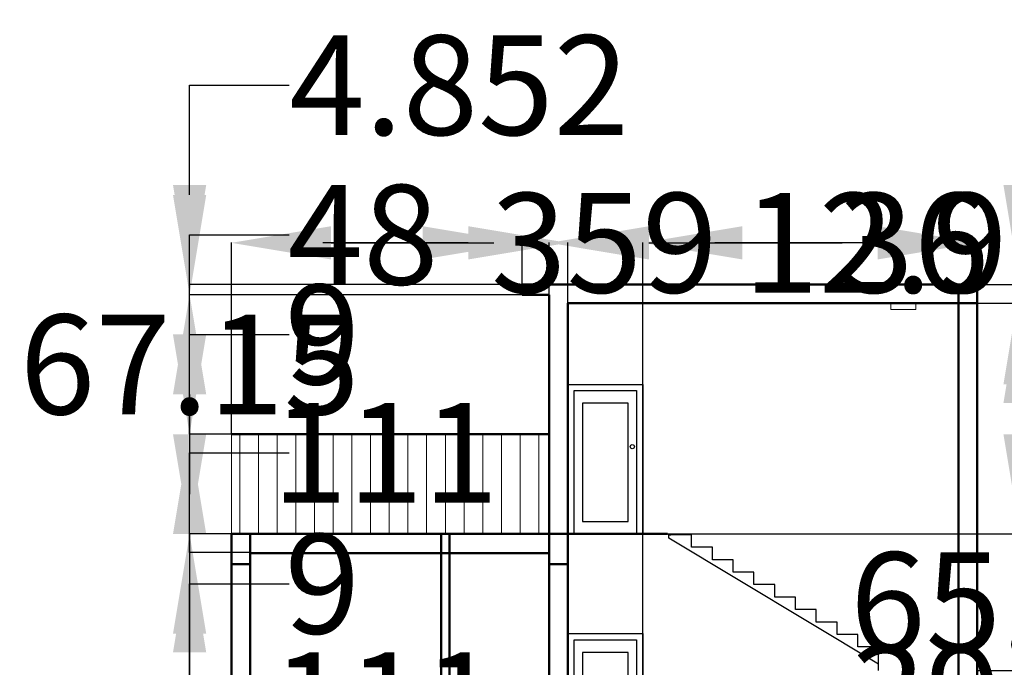
# Model space of a CAD drawing. Units: inches. Extents: x 131 to 858, y -65 to 554.
# Tile 3 of 4: x 131 to 605, y 242 to 554. Entities that reach past the tile are written whole.
import ezdxf

# ---------------------------------------------------------------- set-up
doc = ezdxf.new("R2010")
doc.units = ezdxf.units.IN
doc.header["$MEASUREMENT"] = 0
for name, color, linetype, lineweight in [('A-ANNO-DIMS', 2, 'Continuous', 18), ('A-DOOR', 4, 'Continuous', 25), ('A-EQPM', 8, 'Continuous', 18), ('A-FLOR-HRAL', 4, 'Continuous', 18), ('A-FLOR-STRS', 3, 'Continuous', 25), ('A-SECT', 7, 'Continuous', 50)]:
    doc.layers.add(name, color=color, linetype=linetype, lineweight=lineweight)
doc.styles.get("Standard").update_dxf_attribs({"font": 'arial.ttf'})
doc.dimstyles.get("Standard").update_dxf_attribs({"dimtxt": 48, "dimasz": 48, "dimexe": 0.18, "dimexo": 0.0625, "dimgap": 0.09, "dimtad": 0, "dimtih": 1, "dimtoh": 1, "dimdec": 0, "dimrnd": 72, "dimzin": 0, "dimdsep": 46, "dimlunit": 3, "dimtxsty": 'Standard', "dimcen": 0.09, "dimadec": 0, "dimazin": 0, "dimtfac": 1, "dimtdec": 0, "dimtofl": 0, "dimtmove": 0, "dimatfit": 3, "dimfxl": 1, "dimtolj": 1, "dimtzin": 0, "dimarcsym": 0})

# ---------------------------------------------------------------- blocks, each defined once
blk = doc.blocks.new('*U3')
blk.add_lwpolyline([(3.12, 0.01), (0.12, 0.01), (0.12, 72.01), (36.12, 72.01), (36.12, 0.01), (33.12, 0.01)])
for points in [[(33.12, 68.99), (33.12, 0.01), (3.12, 0.01), (3.12, 68.99)], [(29.12, 6.01), (29.12, 62.99), (7.12, 62.99), (7.12, 6.01)]]:
    blk.add_lwpolyline(points, close=True)
blk.add_circle((31.12, 42.01), 1)
blk = doc.blocks.new('*D4')
at = {"layer": 'A-ANNO-DIMS', "color": 0, "lineweight": -2, "transparency": 16777216}
for p, q in [((233.01, 354.61), (233.01, 446.83)), ((281.01, 446.65), (359.38, 446.65)), ((544.04, 446.65), (465.68, 446.65)), ((592.04, 426.61), (592.04, 446.83))]:
    blk.add_line(p, q, dxfattribs=at)
at = {"layer": 'A-ANNO-DIMS', "color": 0, "transparency": 16777216}
for points in [[(281.01, 454.65), (281.01, 438.65), (233.01, 446.65)], [(544.04, 454.65), (544.04, 438.65), (592.04, 446.65)]]:
    blk.add_solid(points, dxfattribs=at)
at = {"layer": 'Defpoints', "color": 0, "transparency": 16777216}
for p in [(592.04, 446.65), (592.04, 426.55), (233.01, 354.55)]:
    blk.add_point(p, dxfattribs=at)
at = {"layer": 'A-ANNO-DIMS', "color": 0, "transparency": 16777216, "insert": (412.53, 446.65), "char_height": 48, "attachment_point": 5}
blk.add_mtext('\\A1;359', dxfattribs=at)
blk = doc.blocks.new('*D5')
at = {"layer": 'A-ANNO-DIMS', "color": 0, "lineweight": -2, "transparency": 16777216}
for p, q in [((325.03, 446.65), (277.03, 446.65)), ((373.03, 426.61), (373.03, 446.83)), ((386.01, 421.76), (386.01, 446.83)), ((434.01, 446.65), (482.01, 446.65))]:
    blk.add_line(p, q, dxfattribs=at)
at = {"layer": 'A-ANNO-DIMS', "color": 0, "transparency": 16777216}
for points in [[(325.03, 454.65), (325.03, 438.65), (373.03, 446.65)], [(434.01, 454.65), (434.01, 438.65), (386.01, 446.65)]]:
    blk.add_solid(points, dxfattribs=at)
at = {"layer": 'Defpoints', "color": 0, "transparency": 16777216}
for p in [(386.01, 446.65), (373.03, 426.55), (386.01, 421.7)]:
    blk.add_point(p, dxfattribs=at)
at = {"layer": 'A-ANNO-DIMS', "color": 0, "transparency": 16777216, "insert": (579.38, 446.65), "char_height": 48, "attachment_point": 5}
blk.add_mtext('\\A1;12.984', dxfattribs=at)
blk = doc.blocks.new('*D14')
at = {"layer": 'A-ANNO-DIMS', "color": 0, "lineweight": -2, "transparency": 16777216}
for p, q in [((592.11, 426.55), (612.82, 426.55)), ((612.64, 378.55), (612.64, 253.56)), ((612.64, 79.34), (612.64, 204.33)), ((233.08, 31.34), (612.82, 31.34))]:
    blk.add_line(p, q, dxfattribs=at)
at = {"layer": 'A-ANNO-DIMS', "color": 0, "transparency": 16777216}
for points in [[(604.64, 378.55), (620.64, 378.55), (612.64, 426.55)], [(604.64, 79.34), (620.64, 79.34), (612.64, 31.34)]]:
    blk.add_solid(points, dxfattribs=at)
at = {"layer": 'Defpoints', "color": 0, "transparency": 16777216}
for p in [(592.04, 426.55), (612.64, 426.55), (233.01, 31.34)]:
    blk.add_point(p, dxfattribs=at)
at = {"layer": 'A-ANNO-DIMS', "color": 0, "transparency": 16777216, "insert": (612.64, 228.94), "char_height": 48, "attachment_point": 5}
blk.add_mtext('\\A1;395.2', dxfattribs=at)
blk = doc.blocks.new('*D23')
at = {"layer": 'A-ANNO-DIMS', "color": 0, "lineweight": -2, "transparency": 16777216}
for p, q in [((212.91, 177.55), (212.91, 225.55)), ((212.91, 225.55), (260.91, 225.55)), ((241.95, 177.55), (212.73, 177.55)), ((212.91, 114.55), (212.91, 129.55)), ((232.95, 66.55), (212.73, 66.55))]:
    blk.add_line(p, q, dxfattribs=at)
at = {"layer": 'A-ANNO-DIMS', "color": 0, "transparency": 16777216}
for points in [[(204.91, 129.55), (220.91, 129.55), (212.91, 177.55)], [(204.91, 114.55), (220.91, 114.55), (212.91, 66.55)]]:
    blk.add_solid(points, dxfattribs=at)
at = {"layer": 'Defpoints', "color": 0, "transparency": 16777216}
for p in [(212.91, 177.55), (242.01, 177.55), (233.01, 66.55)]:
    blk.add_point(p, dxfattribs=at)
at = {"layer": 'A-ANNO-DIMS', "color": 0, "transparency": 16777216, "insert": (307.14, 225.55), "char_height": 48, "attachment_point": 5}
blk.add_mtext('\\A1;111', dxfattribs=at)
blk = doc.blocks.new('*D24')
at = {"layer": 'A-ANNO-DIMS', "color": 0, "lineweight": -2, "transparency": 16777216}
for p, q in [((212.91, 234.55), (212.91, 282.55)), ((212.91, 282.55), (260.91, 282.55)), ((232.95, 186.55), (212.73, 186.55)), ((241.95, 177.55), (212.73, 177.55)), ((212.91, 129.55), (212.91, 81.55))]:
    blk.add_line(p, q, dxfattribs=at)
at = {"layer": 'A-ANNO-DIMS', "color": 0, "transparency": 16777216}
for points in [[(204.91, 234.55), (220.91, 234.55), (212.91, 186.55)], [(204.91, 129.55), (220.91, 129.55), (212.91, 177.55)]]:
    blk.add_solid(points, dxfattribs=at)
at = {"layer": 'Defpoints', "color": 0, "transparency": 16777216}
for p in [(212.91, 186.55), (233.01, 186.55), (242.01, 177.55)]:
    blk.add_point(p, dxfattribs=at)
at = {"layer": 'A-ANNO-DIMS', "color": 0, "transparency": 16777216, "insert": (276.79, 282.55), "char_height": 48, "attachment_point": 5}
blk.add_mtext('\\A1;9', dxfattribs=at)
blk = doc.blocks.new('*D25')
at = {"layer": 'A-ANNO-DIMS', "color": 0, "lineweight": -2, "transparency": 16777216}
for p, q in [((212.91, 297.55), (212.91, 345.55)), ((212.91, 345.55), (260.91, 345.55)), ((241.95, 297.55), (212.73, 297.55)), ((212.91, 234.55), (212.91, 249.55)), ((232.95, 186.55), (212.73, 186.55))]:
    blk.add_line(p, q, dxfattribs=at)
at = {"layer": 'A-ANNO-DIMS', "color": 0, "transparency": 16777216}
for points in [[(204.91, 249.55), (220.91, 249.55), (212.91, 297.55)], [(204.91, 234.55), (220.91, 234.55), (212.91, 186.55)]]:
    blk.add_solid(points, dxfattribs=at)
at = {"layer": 'Defpoints', "color": 0, "transparency": 16777216}
for p in [(212.91, 297.55), (242.01, 297.55), (233.01, 186.55)]:
    blk.add_point(p, dxfattribs=at)
at = {"layer": 'A-ANNO-DIMS', "color": 0, "transparency": 16777216, "insert": (307.14, 345.55), "char_height": 48, "attachment_point": 5}
blk.add_mtext('\\A1;111', dxfattribs=at)
blk = doc.blocks.new('*D26')
at = {"layer": 'A-ANNO-DIMS', "color": 0, "lineweight": -2, "transparency": 16777216}
for p, q in [((212.91, 354.55), (212.91, 402.55)), ((212.91, 402.55), (260.91, 402.55)), ((232.95, 306.55), (212.73, 306.55)), ((241.95, 297.55), (212.73, 297.55)), ((212.91, 249.55), (212.91, 201.55))]:
    blk.add_line(p, q, dxfattribs=at)
at = {"layer": 'A-ANNO-DIMS', "color": 0, "transparency": 16777216}
for points in [[(204.91, 354.55), (220.91, 354.55), (212.91, 306.55)], [(204.91, 249.55), (220.91, 249.55), (212.91, 297.55)]]:
    blk.add_solid(points, dxfattribs=at)
at = {"layer": 'Defpoints', "color": 0, "transparency": 16777216}
for p in [(212.91, 306.55), (233.01, 306.55), (242.01, 297.55)]:
    blk.add_point(p, dxfattribs=at)
at = {"layer": 'A-ANNO-DIMS', "color": 0, "transparency": 16777216, "insert": (276.79, 402.55), "char_height": 48, "attachment_point": 5}
blk.add_mtext('\\A1;9', dxfattribs=at)
blk = doc.blocks.new('*D27')
at = {"layer": 'A-ANNO-DIMS', "color": 0, "lineweight": -2, "transparency": 16777216}
for p, q in [((212.91, 402.55), (212.91, 450.55)), ((212.91, 450.55), (260.91, 450.55)), ((232.95, 354.55), (212.73, 354.55)), ((232.95, 306.55), (212.73, 306.55)), ((212.91, 258.55), (212.91, 210.55))]:
    blk.add_line(p, q, dxfattribs=at)
at = {"layer": 'A-ANNO-DIMS', "color": 0, "transparency": 16777216}
for points in [[(204.91, 402.55), (220.91, 402.55), (212.91, 354.55)], [(204.91, 258.55), (220.91, 258.55), (212.91, 306.55)]]:
    blk.add_solid(points, dxfattribs=at)
at = {"layer": 'Defpoints', "color": 0, "transparency": 16777216}
for p in [(212.91, 354.55), (233.01, 354.55), (233.01, 306.55)]:
    blk.add_point(p, dxfattribs=at)
at = {"layer": 'A-ANNO-DIMS', "color": 0, "transparency": 16777216, "insert": (296.4, 450.55), "char_height": 48, "attachment_point": 5}
blk.add_mtext('\\A1;48', dxfattribs=at)
blk = doc.blocks.new('*D28')
at = {"layer": 'A-ANNO-DIMS', "color": 0, "lineweight": -2, "transparency": 16777216}
for p, q in [((212.914446, 469.69966), (212.914446, 517.69966)), ((372.967658, 421.69966), (212.734446, 421.69966)), ((232.951946, 354.551418), (212.734446, 354.551418)), ((212.914446, 306.551418), (212.914446, 258.551418))]:
    blk.add_line(p, q, dxfattribs=at)
at = {"layer": 'A-ANNO-DIMS', "color": 0, "transparency": 16777216}
for points in [[(204.914446, 469.69966), (220.914446, 469.69966), (212.914446, 421.69966)], [(204.914446, 306.551418), (220.914446, 306.551418), (212.914446, 354.551418)]]:
    blk.add_solid(points, dxfattribs=at)
at = {"layer": 'Defpoints', "color": 0, "transparency": 16777216}
for p in [(212.914446, 421.69966), (373.030158, 421.69966), (233.014446, 354.551418)]:
    blk.add_point(p, dxfattribs=at)
at = {"layer": 'A-ANNO-DIMS', "color": 0, "transparency": 16777216, "insert": (212.914446, 388.125539), "char_height": 48, "attachment_point": 5}
blk.add_mtext('\\A1;67.15', dxfattribs=at)
blk = doc.blocks.new('*D29')
at = {"layer": 'A-ANNO-DIMS', "color": 0, "lineweight": -2, "transparency": 16777216}
for p, q in [((212.91, 474.55), (212.91, 522.55)), ((212.91, 522.55), (260.91, 522.55)), ((372.97, 426.55), (212.73, 426.55)), ((372.97, 421.7), (212.73, 421.7)), ((212.91, 373.7), (212.91, 325.7))]:
    blk.add_line(p, q, dxfattribs=at)
at = {"layer": 'A-ANNO-DIMS', "color": 0, "transparency": 16777216}
for points in [[(204.91, 474.55), (220.91, 474.55), (212.91, 426.55)], [(204.91, 373.7), (220.91, 373.7), (212.91, 421.7)]]:
    blk.add_solid(points, dxfattribs=at)
at = {"layer": 'Defpoints', "color": 0, "transparency": 16777216}
for p in [(212.91, 426.55), (373.03, 426.55), (373.03, 421.7)]:
    blk.add_point(p, dxfattribs=at)
at = {"layer": 'A-ANNO-DIMS', "color": 0, "transparency": 16777216, "insert": (342.71, 522.55), "char_height": 48, "attachment_point": 5}
blk.add_mtext('\\A1;4.852', dxfattribs=at)
blk = doc.blocks.new('*D30')
at = {"layer": 'A-ANNO-DIMS', "color": 0, "lineweight": -2, "transparency": 16777216}
for p, q in [((612.64, 417.55), (612.64, 465.55)), ((612.64, 465.55), (660.64, 465.55)), ((592.11, 417.55), (612.82, 417.55)), ((612.64, 354.55), (612.64, 369.55)), ((443.08, 306.55), (612.82, 306.55))]:
    blk.add_line(p, q, dxfattribs=at)
at = {"layer": 'A-ANNO-DIMS', "color": 0, "transparency": 16777216}
for points in [[(604.64, 369.55), (620.64, 369.55), (612.64, 417.55)], [(604.64, 354.55), (620.64, 354.55), (612.64, 306.55)]]:
    blk.add_solid(points, dxfattribs=at)
at = {"layer": 'Defpoints', "color": 0, "transparency": 16777216}
for p in [(592.04, 417.55), (612.64, 417.55), (443.01, 306.55)]:
    blk.add_point(p, dxfattribs=at)
at = {"layer": 'A-ANNO-DIMS', "color": 0, "transparency": 16777216, "insert": (706.86, 465.55), "char_height": 48, "attachment_point": 5}
blk.add_mtext('\\A1;111', dxfattribs=at)
blk = doc.blocks.new('*D31')
at = {"layer": 'A-ANNO-DIMS', "color": 0, "lineweight": -2, "transparency": 16777216}
for p, q in [((612.64, 474.55), (612.64, 522.55)), ((612.64, 522.55), (660.64, 522.55)), ((592.11, 426.55), (612.82, 426.55)), ((592.11, 417.55), (612.82, 417.55)), ((612.64, 369.55), (612.64, 321.55))]:
    blk.add_line(p, q, dxfattribs=at)
at = {"layer": 'A-ANNO-DIMS', "color": 0, "transparency": 16777216}
for points in [[(604.64, 474.55), (620.64, 474.55), (612.64, 426.55)], [(604.64, 369.55), (620.64, 369.55), (612.64, 417.55)]]:
    blk.add_solid(points, dxfattribs=at)
at = {"layer": 'Defpoints', "color": 0, "transparency": 16777216}
for p in [(592.04, 426.55), (612.64, 426.55), (592.04, 417.55)]:
    blk.add_point(p, dxfattribs=at)
at = {"layer": 'A-ANNO-DIMS', "color": 0, "transparency": 16777216, "insert": (676.51, 522.55), "char_height": 48, "attachment_point": 5}
blk.add_mtext('\\A1;9', dxfattribs=at)
blk = doc.blocks.new('*D32')
at = {"layer": 'A-ANNO-DIMS', "color": 0, "lineweight": -2, "transparency": 16777216}
for p, q in [((347.01, 446.65), (299.01, 446.65)), ((395.01, 138.61), (395.01, 446.83)), ((431.01, 138.61), (431.01, 446.83)), ((479.01, 446.65), (527.01, 446.65))]:
    blk.add_line(p, q, dxfattribs=at)
at = {"layer": 'A-ANNO-DIMS', "color": 0, "transparency": 16777216}
for points in [[(347.01, 454.65), (347.01, 438.65), (395.01, 446.65)], [(479.01, 454.65), (479.01, 438.65), (431.01, 446.65)]]:
    blk.add_solid(points, dxfattribs=at)
at = {"layer": 'Defpoints', "color": 0, "transparency": 16777216}
for p in [(431.01, 446.65), (395.01, 138.55), (431.01, 138.55)]:
    blk.add_point(p, dxfattribs=at)
at = {"layer": 'A-ANNO-DIMS', "color": 0, "transparency": 16777216, "insert": (561.45, 446.65), "char_height": 48, "attachment_point": 5}
blk.add_mtext('\\A1;36', dxfattribs=at)
blk = doc.blocks.new('*D42')
at = {"layer": 'A-ANNO-DIMS', "color": 0, "lineweight": -2, "transparency": 16777216}
for p, q in [((612.64, 240.89), (612.64, 288.89)), ((612.64, 288.89), (660.64, 288.89)), ((592.6, 240.89), (612.82, 240.89)), ((612.64, 174.36), (612.64, 192.89)), ((592.11, 126.36), (612.82, 126.36))]:
    blk.add_line(p, q, dxfattribs=at)
at = {"layer": 'A-ANNO-DIMS', "color": 0, "transparency": 16777216}
for points in [[(604.64, 192.89), (620.64, 192.89), (612.64, 240.89)], [(604.64, 174.36), (620.64, 174.36), (612.64, 126.36)]]:
    blk.add_solid(points, dxfattribs=at)
at = {"layer": 'Defpoints', "color": 0, "transparency": 16777216}
for p in [(592.54, 240.89), (612.64, 240.89), (592.04, 126.36)]:
    blk.add_point(p, dxfattribs=at)
at = {"layer": 'A-ANNO-DIMS', "color": 0, "transparency": 16777216, "insert": (758.11, 288.89), "char_height": 48, "attachment_point": 5}
blk.add_mtext('\\A1;114.53', dxfattribs=at)
blk = doc.blocks.new('*D43')
at = {"layer": 'A-ANNO-DIMS', "color": 0, "lineweight": -2, "transparency": 16777216}
for p, q in [((612.639956, 354.551418), (612.639956, 402.551418)), ((443.076946, 306.551418), (612.819956, 306.551418)), ((592.602456, 240.886672), (612.819956, 240.886672)), ((612.639956, 192.886672), (612.639956, 144.886672))]:
    blk.add_line(p, q, dxfattribs=at)
at = {"layer": 'A-ANNO-DIMS', "color": 0, "transparency": 16777216}
for points in [[(604.639956, 354.551418), (620.639956, 354.551418), (612.639956, 306.551418)], [(604.639956, 192.886672), (620.639956, 192.886672), (612.639956, 240.886672)]]:
    blk.add_solid(points, dxfattribs=at)
at = {"layer": 'Defpoints', "color": 0, "transparency": 16777216}
for p in [(443.014446, 306.551418), (612.639956, 306.551418), (592.539956, 240.886672)]:
    blk.add_point(p, dxfattribs=at)
at = {"layer": 'A-ANNO-DIMS', "color": 0, "transparency": 16777216, "insert": (612.639956, 273.719045), "char_height": 48, "attachment_point": 5}
blk.add_mtext('\\A1;65.66', dxfattribs=at)

msp = doc.modelspace()

# ---------------------------------------------------------------- linework, layer by layer
at = {"layer": 'A-EQPM'}
msp.add_lwpolyline([(562.4065, 417.5514), (550.4054, 417.5514), (550.4054, 414.5757), (562.4065, 414.5757)], close=True, dxfattribs=at)
at = {"layer": 'A-FLOR-HRAL'}
for p, q in [((233.0144, 306.5514), (233.0144, 354.5514)), ((233.0144, 354.5514), (233.0144, 306.5514)), ((237.0144, 354.5514), (237.0144, 306.5514)), ((246.0144, 354.5514), (246.0144, 306.5514)), ((255.0144, 354.5514), (255.0144, 306.5514)), ((264.0144, 354.5514), (264.0144, 306.5514)), ((273.0144, 354.5514), (273.0144, 306.5514)), ((282.0144, 354.5514), (282.0144, 306.5514)), ((291.0144, 354.5514), (291.0144, 306.5514)), ((300.0144, 354.5514), (300.0144, 306.5514)), ((309.0144, 354.5514), (309.0144, 306.5514)), ((318.0144, 354.5514), (318.0144, 306.5514)), ((327.0144, 354.5514), (327.0144, 306.5514)), ((336.0144, 354.5514), (336.0144, 306.5514)), ((345.0144, 354.5514), (345.0144, 306.5514)), ((354.0144, 354.5514), (354.0144, 306.5514)), ((363.0144, 354.5514), (363.0144, 306.5514)), ((372.0144, 354.5514), (372.0144, 306.5514)), ((381.0144, 354.5514), (381.0144, 306.5514))]:
    msp.add_line(p, q, dxfattribs=at)
at = {"layer": 'A-FLOR-STRS'}
for p, q in [((443.511, 304.4472), (443.511, 306.1622)), ((443.511, 306.1622), (444.54, 306.1622)), ((544.54, 243.8298), (443.511, 304.4472)), ((454.54, 306.1622), (444.54, 306.1622)), ((454.54, 300.1622), (454.54, 306.1622)), ((454.54, 306.1622), (454.54, 306.1622)), ((464.54, 300.1622), (454.54, 300.1622)), ((464.54, 294.1622), (464.54, 300.1622)), ((464.54, 300.1622), (464.54, 300.1622)), ((474.54, 294.1622), (464.54, 294.1622)), ((474.54, 288.1622), (474.54, 294.1622)), ((474.54, 294.1622), (474.54, 294.1622)), ((484.54, 288.1622), (474.54, 288.1622)), ((484.54, 282.1622), (484.54, 288.1622)), ((484.54, 288.1622), (484.54, 288.1622)), ((494.54, 282.1622), (484.54, 282.1622)), ((494.54, 276.1622), (494.54, 282.1622)), ((494.54, 282.1622), (494.54, 282.1622)), ((504.54, 276.1622), (494.54, 276.1622)), ((504.54, 270.1622), (504.54, 276.1622)), ((504.54, 276.1622), (504.54, 276.1622)), ((514.54, 270.1622), (504.54, 270.1622)), ((514.54, 264.1622), (514.54, 270.1622)), ((514.54, 270.1622), (514.54, 270.1622)), ((524.54, 264.1622), (514.54, 264.1622)), ((524.54, 258.1622), (524.54, 264.1622)), ((524.54, 264.1622), (524.54, 264.1622)), ((534.54, 258.1622), (524.54, 258.1622)), ((534.54, 252.1622), (534.54, 258.1622)), ((534.54, 258.1622), (534.54, 258.1622)), ((544.54, 252.1622), (534.54, 252.1622)), ((544.54, 246.1622), (544.54, 252.1622)), ((544.54, 252.1622), (544.54, 252.1622)), ((544.54, 240.8867), (544.54, 246.1622))]:
    msp.add_line(p, q, dxfattribs=at)
at = {"layer": 'A-SECT'}
for p, q in [((373.0302, 421.6997), (373.0302, 426.5514)), ((373.0302, 426.5514), (386.0144, 426.5514)), ((386.0144, 426.5514), (592.0434, 426.5514)), ((583.0434, 126.3568), (583.0434, 426.5514)), ((592.0434, 126.3568), (592.0434, 426.5514)), ((386.0144, 421.6997), (373.0302, 421.6997)), ((386.0144, 306.5514), (386.0144, 421.6997)), ((395.0144, 306.5514), (395.0144, 417.5514)), ((395.0144, 417.5514), (592.0434, 417.5514)), ((395.0144, 48.1342), (395.0144, 366.3568)), ((386.0144, 354.5514), (233.0144, 354.5514)), ((386.0144, 48.1342), (386.0144, 354.5514)), ((233.0144, 292.0345), (233.0144, 306.5514)), ((233.0144, 306.5514), (395.0144, 306.5514)), ((233.0144, 306.5514), (233.0144, 292.0345)), ((233.0144, 292.0345), (233.0144, 306.5514)), ((233.0144, 306.5514), (242.0144, 306.5514)), ((233.0144, 306.5514), (395.0144, 306.5514)), ((233.0144, 306.5514), (233.0144, 57.5514)), ((242.0144, 306.5514), (242.0144, 292.0345)), ((242.0144, 306.5514), (242.0144, 297.5514)), ((242.0144, 306.5514), (242.0144, 297.5514)), ((242.0144, 306.5514), (242.0144, 66.5514)), ((334.0144, 306.5514), (334.0144, 66.5514)), ((338.0144, 306.5514), (338.0144, 297.3694)), ((338.0144, 306.5514), (338.0144, 66.5514)), ((386.0144, 306.5514), (386.0144, 292.0345)), ((386.0144, 292.0345), (386.0144, 306.5514)), ((386.0144, 292.0345), (386.0144, 306.5514)), ((386.0144, 306.5514), (395.0144, 306.5514)), ((386.0144, 306.5514), (386.0144, 66.5514)), ((395.0144, 306.5514), (395.0144, 297.5514)), ((395.0144, 306.5514), (395.0144, 292.0345)), ((395.0144, 306.5514), (395.0144, 297.5514)), ((395.0144, 306.5514), (395.0144, 57.5514)), ((395.0144, 306.5514), (443.0144, 306.5514)), ((242.0144, 297.3694), (386.0144, 297.3694)), ((242.0144, 292.0345), (233.0144, 292.0345)), ((395.0144, 292.0345), (386.0144, 292.0345))]:
    msp.add_line(p, q, dxfattribs=at)

# ---------------------------------------------------------------- block references
at = {"layer": 'A-DOOR'}
for p in [(394.8907, 306.5387), (394.8907, 186.5387)]:
    msp.add_blockref('*U3', p, dxfattribs=at)

# ---------------------------------------------------------------- dimensions: what is measured, and where the dimension line sits
at = {"layer": 'A-ANNO-DIMS'}
for base, p1, p2, override, picture, middle in [((212.9144, 426.5514), (373.0302, 421.6997), (373.0302, 426.5514), {"dimdec": 3, "dimlfac": 1, "dimrnd": 0, "dimzin": 0, "dimdsep": 46, "dimlunit": 2}, '*D29', (342.7125, 522.5514)), ((612.64, 426.5514), (592.0434, 417.5514), (592.0434, 426.5514), {"dimdec": 0, "dimlfac": 1, "dimrnd": 0, "dimzin": 0, "dimdsep": 46, "dimlunit": 2}, '*D31', (676.5117, 522.5514)), ((212.9144, 421.6997), (233.0144, 354.5514), (373.0302, 421.6997), {"dimdec": 2, "dimlfac": 1, "dimrnd": 0, "dimzin": 0, "dimdsep": 46, "dimlunit": 2}, '*D28', (212.9144, 388.1255)), ((612.64, 417.5514), (443.0144, 306.5514), (592.0434, 417.5514), {"dimdec": 0, "dimlfac": 1, "dimrnd": 0, "dimzin": 0, "dimdsep": 46, "dimlunit": 2}, '*D30', (706.8637, 465.5514)), ((212.9144, 354.5514), (233.0144, 306.5514), (233.0144, 354.5514), {"dimdec": 0, "dimlfac": 1, "dimrnd": 0, "dimzin": 0, "dimdsep": 46, "dimlunit": 2}, '*D27', (296.3987, 450.5514)), ((212.9144, 306.5514), (242.0144, 297.5514), (233.0144, 306.5514), {"dimdec": 0, "dimlfac": 1, "dimrnd": 0, "dimzin": 0, "dimdsep": 46, "dimlunit": 2}, '*D26', (276.7862, 402.5514)), ((612.64, 426.5514), (233.0144, 31.336), (592.0434, 426.5514), {"dimdec": 1, "dimlfac": 1, "dimrnd": 0, "dimzin": 0, "dimdsep": 46, "dimlunit": 2}, '*D14', (612.64, 228.9437)), ((612.64, 306.5514), (592.54, 240.8867), (443.0144, 306.5514), {"dimdec": 2, "dimlfac": 1, "dimrnd": 0, "dimzin": 0, "dimdsep": 46, "dimlunit": 2}, '*D43', (612.64, 273.719)), ((212.9144, 297.5514), (233.0144, 186.5514), (242.0144, 297.5514), {"dimdec": 0, "dimlfac": 1, "dimrnd": 0, "dimzin": 0, "dimdsep": 46, "dimlunit": 2}, '*D25', (307.1381, 345.5514)), ((612.64, 240.8867), (592.0434, 126.3568), (592.54, 240.8867), {"dimdec": 2, "dimlfac": 1, "dimrnd": 0, "dimzin": 0, "dimdsep": 46, "dimlunit": 2}, '*D42', (758.1051, 288.8867)), ((212.9144, 186.5514), (242.0144, 177.5514), (233.0144, 186.5514), {"dimdec": 0, "dimlfac": 1, "dimrnd": 0, "dimzin": 0, "dimdsep": 46, "dimlunit": 2}, '*D24', (276.7862, 282.5514)), ((212.9144, 177.5514), (233.0144, 66.5514), (242.0144, 177.5514), {"dimdec": 0, "dimlfac": 1, "dimrnd": 0, "dimzin": 0, "dimdsep": 46, "dimlunit": 2}, '*D23', (307.1381, 225.5514))]:
    dim = msp.add_linear_dim(base=base, p1=p1, p2=p2, angle=90, dimstyle='Standard', override=override, dxfattribs=at)
    dim.commit()
    dim.dimension.update_dxf_attribs({"geometry": picture, "text_midpoint": middle})
for base, p1, p2, override, picture, middle in [((592.0434, 446.6514), (233.0144, 354.5514), (592.0434, 426.5514), {"dimdec": 0, "dimlfac": 1, "dimrnd": 0, "dimzin": 0, "dimdsep": 46, "dimlunit": 2}, '*D4', (412.5289, 446.6514)), ((386.0144, 446.6514), (373.0302, 426.5514), (386.0144, 421.6997), {"dimdec": 3, "dimlfac": 1, "dimrnd": 0, "dimzin": 0, "dimdsep": 46, "dimlunit": 2}, '*D5', (579.3814, 446.6514)), ((431.0144, 446.6514), (395.0144, 138.5514), (431.0144, 138.5514), {"dimdec": 0, "dimlfac": 1, "dimrnd": 0, "dimzin": 0, "dimdsep": 46, "dimlunit": 2}, '*D32', (561.451, 446.6514))]:
    dim = msp.add_linear_dim(base=base, p1=p1, p2=p2, dimstyle='Standard', override=override, dxfattribs=at)
    dim.commit()
    dim.dimension.update_dxf_attribs({"geometry": picture, "text_midpoint": middle})

doc.saveas('drawing.dxf')
